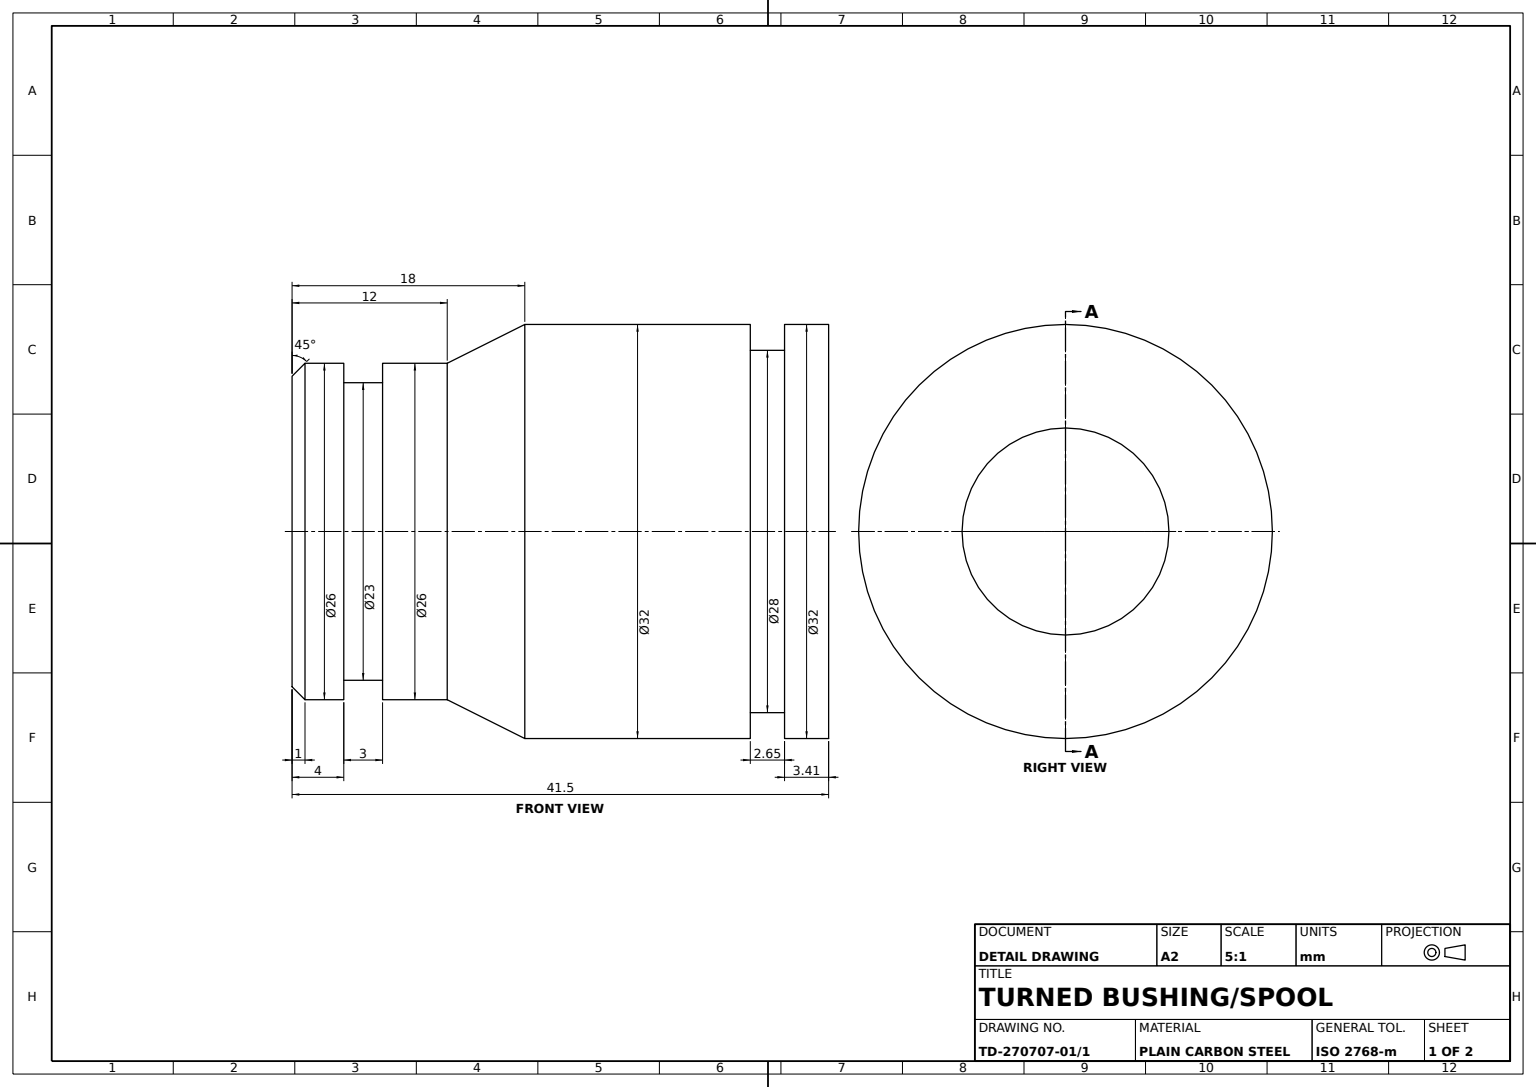
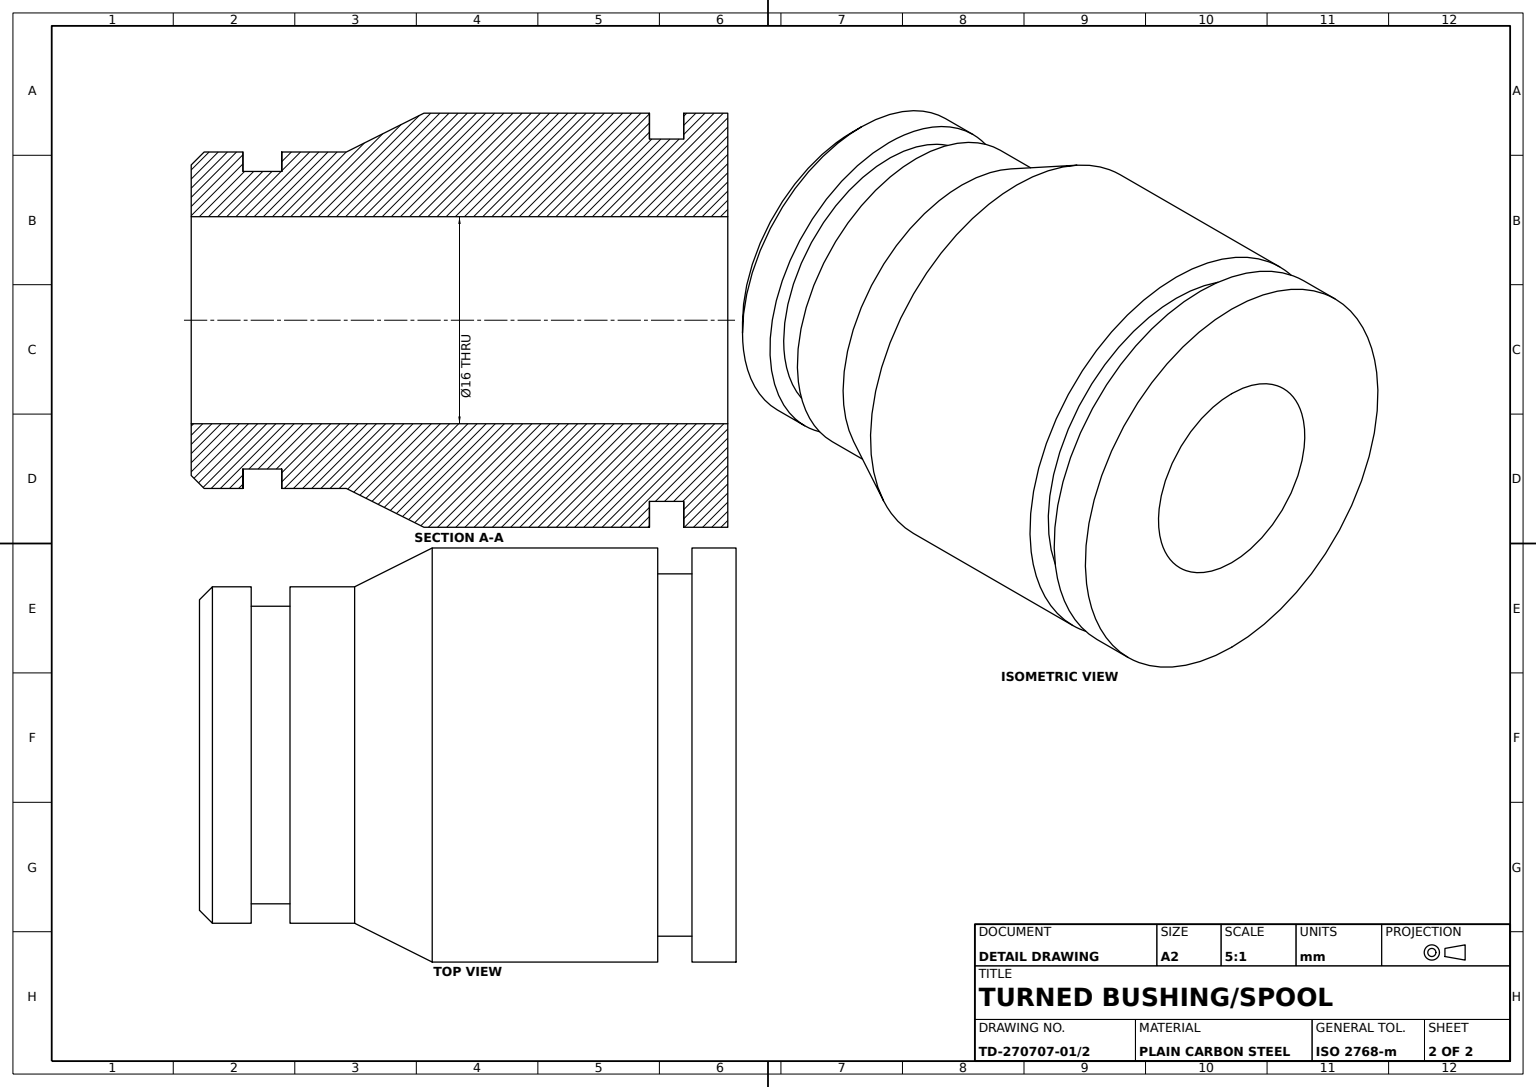
SolidWorks part; units mm, degrees
material "Plain Carbon Steel"
ref_plane "Front Plane" through (0, 0, 0) normal (0, 0, 1) x (1, 0, 0)
ref_plane "Top Plane" through (0, 0, 0) normal (0, 1, 0) x (1, 0, 0)
ref_plane "Right Plane" through (0, 0, 0) normal (1, 0, 0) x (0, 0, -1)
sketch "Bushing Profile Sketch" plane through (0, 0, 0) normal (0, 0, 1) x (1, 0, 0)
  line L0 (-43.7918, 0) -> (43.7918, 0) construction
  line L1 (-9.5974, 8) -> (31.9026, 8)
  line L2 (31.9026, 8) -> (31.9026, 16)
  line L3 (31.9026, 16) -> (28.4931, 16)
  line L4 (28.4931, 16) -> (28.4931, 14)
  line L5 (28.4931, 14) -> (25.8439, 14)
  line L6 (25.8439, 14) -> (25.8439, 16)
  line L7 (25.8439, 16) -> (8.4026, 16)
  line L8 (8.4026, 16) -> (2.4026, 13)
  line L9 (2.4026, 13) -> (-8.5974, 13)
  line L10 (-9.5974, 12) -> (-9.5974, 8)
  line L11 (-8.5974, 13) -> (-9.5974, 12)
  point P3 (0, 0)
  point P14 (-9.5974, 13)
  dimension "D1" = 8
  dimension "D2" = 16
  dimension "D3" = 14
  dimension "D4" = 12
  dimension "D5" = 16
  dimension "D6" = 41.5
  dimension "D7" = 18
  dimension "D8" = 5
  dimension "D9" = 9.5974
  dimension "D10" = 3.4096
  dimension "D12" = 2.6492
revolve "Bushing Body Revolve" add sketch "Bushing Profile Sketch" angle 360 about L0
sketch "Groove Profile Sketch 3x3" plane through (0, 0, 0) normal (0, 0, 1) x (1, 0, 0)
  line L0 (-8.5974, -13) -> (-8.5974, 13) construction
  line L1 (-5.5974, 15.5441) -> (-2.5974, 15.5441)
  line L2 (-5.5974, 15.5441) -> (-5.5974, 11.4981)
  line L3 (-5.5974, 11.4981) -> (-2.5974, 11.4981)
  line L4 (-2.5974, 15.5441) -> (-2.5974, 11.4981)
  line L5 (-18.3977, 0) -> (36.9536, 0) construction
  dimension "D1" = 3
  dimension "D2" = 3
  dimension "D3" = 11.4981
  dimension "D4" = 15.5441
revolve "Groove Cut 3x3" cut sketch "Groove Profile Sketch 3x3" angle 360 about L5
